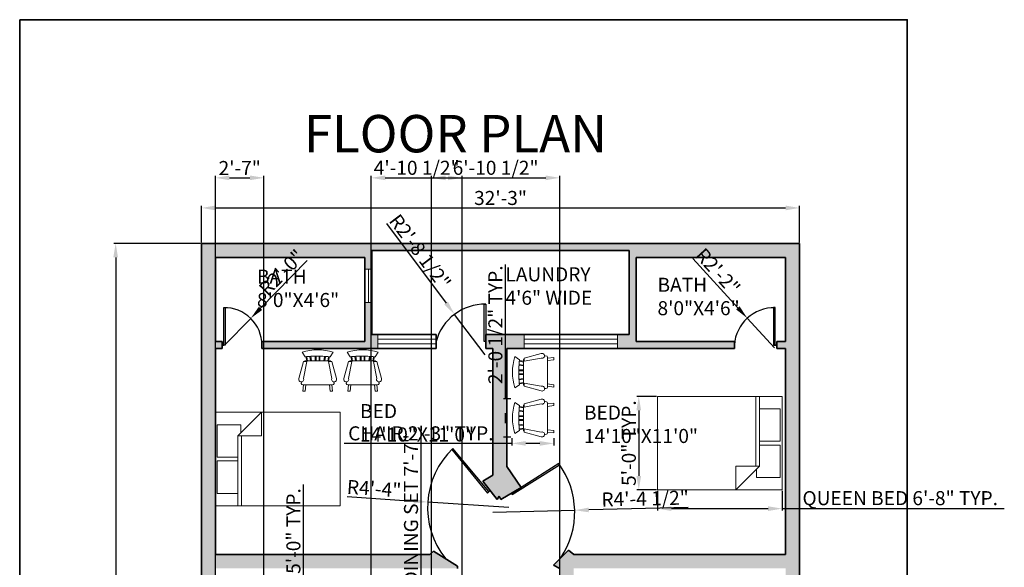
# Model space of a CAD drawing. Units: inches. Extents: x 32476 to 33108, y 58720 to 59630.
# Tile 6 of 6: x 32476 to 33108, y 59278 to 59630. Entities that reach past the tile are written whole.
import ezdxf

# ---------------------------------------------------------------- set-up
doc = ezdxf.new("R2010")
doc.units = ezdxf.units.IN
for name, color, linetype, lineweight in [('A-ANNO-DIMS', 6, 'Continuous', 18), ('A-ANNO-TTLB', 7, 'Continuous', 35), ('A-AREA-IDEN', 32, 'Continuous', 18), ('A-DOOR', 4, 'Continuous', 25), ('A-FURN', 8, 'Continuous', 18), ('A-GLAZ', 4, 'Continuous', 18), ('A-WALL', 7, 'Continuous', 35), ('A-WALL-PATT', 251, 'Continuous', 13)]:
    doc.layers.add(name, color=color, linetype=linetype, lineweight=lineweight)
doc.styles.get("Standard").update_dxf_attribs({"font": 'arial.ttf'})
doc.dimstyles.new('ISO-25', dxfattribs={"dimtxt": 9, "dimasz": 9, "dimexe": 1.25, "dimexo": 0.625, "dimtad": 1, "dimdec": 1, "dimrnd": 9, "dimlunit": 3, "dimtxsty": 'Standard', "dimcen": 2.5, "dimadec": 0, "dimazin": 0, "dimtfac": 1, "dimtdec": 1, "dimtmove": 0, "dimatfit": 3, "dimfxl": 1, "dimarcsym": 0})

# ---------------------------------------------------------------- blocks, each defined once
blk = doc.blocks.new('*D1')
at = {"layer": 'A-ANNO-DIMS', "color": 0, "lineweight": -2, "transparency": 16777216}
for p, q in [((32593.04, 59486.84), (32593.04, 59510.18)), ((32602.04, 59508.93), (32968.04, 59508.93)), ((32977.04, 59486.84), (32977.04, 59510.18))]:
    blk.add_line(p, q, dxfattribs=at)
at = {"layer": 'A-ANNO-DIMS', "color": 0, "transparency": 16777216}
for points in [[(32602.04, 59510.43), (32602.04, 59507.43), (32593.04, 59508.93)], [(32968.04, 59510.43), (32968.04, 59507.43), (32977.04, 59508.93)]]:
    blk.add_solid(points, dxfattribs=at)
at = {"layer": 'Defpoints', "color": 0, "transparency": 16777216}
for p in [(32977.04, 59508.93), (32593.04, 59486.22), (32977.04, 59486.22)]:
    blk.add_point(p, dxfattribs=at)
at = {"layer": 'A-ANNO-DIMS', "color": 0, "transparency": 16777216, "insert": (32785.04, 59514.15), "char_height": 9, "attachment_point": 5}
blk.add_mtext('32\'-3"', dxfattribs=at)
blk = doc.blocks.new('*D2')
at = {"layer": 'A-ANNO-DIMS', "color": 0, "lineweight": -2, "transparency": 16777216}
for p, q in [((32592.41, 59486.22), (32536.75, 59486.22)), ((32538, 59477.22), (32538, 58799.22)), ((32592.41, 58790.22), (32536.75, 58790.22))]:
    blk.add_line(p, q, dxfattribs=at)
at = {"layer": 'A-ANNO-DIMS', "color": 0, "transparency": 16777216}
for points in [[(32536.5, 59477.22), (32539.5, 59477.22), (32538, 59486.22)], [(32536.5, 58799.22), (32539.5, 58799.22), (32538, 58790.22)]]:
    blk.add_solid(points, dxfattribs=at)
at = {"layer": 'Defpoints', "color": 0, "transparency": 16777216}
for p in [(32593.04, 59486.22), (32538, 58790.22), (32593.04, 58790.22)]:
    blk.add_point(p, dxfattribs=at)
at = {"layer": 'A-ANNO-DIMS', "color": 0, "transparency": 16777216, "insert": (32532.78, 59138.22), "char_height": 9, "attachment_point": 5, "rotation": 90}
blk.add_mtext('57\'-9"', dxfattribs=at)
blk = doc.blocks.new('Bed - Queen')
for p, q in [((0, -80.00003), (0, 0)), ((0, 0), (59.99999, 0)), ((59.99999, 0), (59.99999, -80.00003)), ((7.99999, -1.2), (28.79998, -1.2)), ((7.99999, -14.4), (7.99999, -1.2)), ((28.79998, -1.2), (28.79998, -14.4)), ((31.19999, -1.2), (51.99999, -1.2)), ((31.19999, -14.4), (31.19999, -1.2)), ((51.99999, -1.2), (51.99999, -16.4)), ((0, -14.4), (44.8, -14.4)), ((44.8, -16.8), (0, -16.8)), ((59.99999, -29.6), (44.8, -14.4)), ((44.8, -14.4), (44.8, -29.6)), ((51.99999, -16.4), (46.79936, -16.4)), ((44.8, -29.6), (59.99999, -29.6)), ((59.99999, -80.00003), (0, -80.00003))]:
    blk.add_line(p, q)
blk = doc.blocks.new('Chair - Rocking')
for p, q in [((-8, -4.5), (-10, -1.5)), ((-7.5, -4.5), (-7, -7)), ((-6.5, -7), (-7.02225, -4.43)), ((-4.5, -7), (-4.96674, -4.19951)), ((-4, -7), (-4.40532, -4.16272)), ((-1.5, -4.05012), (-1.5, -7)), ((-1, -7), (-1, -4.05012)), ((1, -7), (1, -4.04655)), ((1.5, -4.05012), (1.5, -7)), ((4, -7), (4.40187, -4.18694)), ((4.5, -7), (4.96761, -4.19437)), ((6.5, -7), (7, -4.4057)), ((7.5, -4.5), (7, -7)), ((8, -4.5), (10, -1.5)), ((-9, -7.5), (-12, -18.49999)), ((-7, -7.5), (-9, -7.5)), ((-9, -18.49999), (-7, -7.5)), ((-8.23428, -6.99939), (-8.3093, -7.47958)), ((-8.23041, -7), (8.23915, -7)), ((7, -7.5), (9, -7.5)), ((9, -18.49999), (7, -7.5)), ((8.31071, -7.48854), (8.23449, -7.00073)), ((9, -7.5), (12, -18.49999)), ((-10.36644, -20.64523), (-10.5, -21.49999)), ((-9, -22.49999), (-9.5, -26.49999)), ((0, -22.49999), (-9.5, -22.49999)), ((-8, -26.49999), (-7.5, -22.49999)), ((0, -22.49999), (9.5, -22.49999)), ((8, -26.49999), (7.5, -22.49999)), ((9, -22.49999), (9.5, -26.49999)), ((10.5, -21.49999), (10.3575, -20.58798)), ((-9.5, -26.49999), (-8, -26.49999)), ((9.5, -26.49999), (8, -26.49999))]:
    blk.add_line(p, q)
for centre, radius, start, end in [((0, -34.08333), 34.08333, 72.93847, 107.0615), ((0, -68.25004), 64.25, 93.92211, 97.15267), ((0, -68.25004), 64.25, 82.84733, 93.92211), ((-10.5, -18.99999), 1.58114, 161.5651, 18.43495), ((10.5, -18.99999), 1.58114, 161.5651, 18.43495), ((-9.5, -21.49999), 1, 180, 270), ((9.5, -21.49999), 1, 270, 0)]:
    blk.add_arc(centre, radius, start, end)
blk = doc.blocks.new('*D15')
at = {"layer": 'A-ANNO-DIMS', "color": 0, "lineweight": -2, "transparency": 16777216}
for p, q in [((32792.22, 59361.34), (32792.22, 59356.67)), ((32819.22, 59361.34), (32819.22, 59356.67)), ((32792.22, 59357.92), (32684.61, 59357.92)), ((32810.22, 59357.92), (32801.22, 59357.92))]:
    blk.add_line(p, q, dxfattribs=at)
at = {"layer": 'A-ANNO-DIMS', "color": 0, "transparency": 16777216}
for points in [[(32801.22, 59359.42), (32801.22, 59356.42), (32792.22, 59357.92)], [(32810.22, 59359.42), (32810.22, 59356.42), (32819.22, 59357.92)]]:
    blk.add_solid(points, dxfattribs=at)
at = {"layer": 'Defpoints', "color": 0, "transparency": 16777216}
for p in [(32792.22, 59361.97), (32819.22, 59361.97), (32792.22, 59357.92)]:
    blk.add_point(p, dxfattribs=at)
at = {"layer": 'A-ANNO-DIMS', "color": 0, "transparency": 16777216, "insert": (32733.91, 59363.2), "char_height": 9, "attachment_point": 5}
blk.add_mtext('CHAIR 2\'-3" TYP.', dxfattribs=at)
blk = doc.blocks.new('*D16')
at = {"layer": 'A-ANNO-DIMS', "color": 0, "lineweight": -2, "transparency": 16777216}
for p, q in [((32788.17, 59386.4), (32788.17, 59472.64)), ((32791.6, 59386.4), (32786.92, 59386.4)), ((32788.17, 59370.97), (32788.17, 59377.4)), ((32791.6, 59361.97), (32786.92, 59361.97))]:
    blk.add_line(p, q, dxfattribs=at)
at = {"layer": 'A-ANNO-DIMS', "color": 0, "transparency": 16777216}
for points in [[(32786.67, 59377.4), (32789.67, 59377.4), (32788.17, 59386.4)], [(32786.67, 59370.97), (32789.67, 59370.97), (32788.17, 59361.97)]]:
    blk.add_solid(points, dxfattribs=at)
at = {"layer": 'Defpoints', "color": 0, "transparency": 16777216}
for p in [(32788.17, 59386.4), (32792.22, 59386.4), (32792.22, 59361.97)]:
    blk.add_point(p, dxfattribs=at)
at = {"layer": 'A-ANNO-DIMS', "color": 0, "transparency": 16777216, "insert": (32782.89, 59434.02), "char_height": 9, "attachment_point": 5, "rotation": 90}
blk.add_mtext('2\'-0 1/2" TYP.', dxfattribs=at)
blk = doc.blocks.new('*D21')
at = {"layer": 'A-ANNO-DIMS', "color": 0, "lineweight": -2, "transparency": 16777216}
for p, q in [((32885.79, 59327.47), (32885.79, 59314.84)), ((32965.79, 59327.47), (32965.79, 59314.84)), ((32894.79, 59316.09), (32956.79, 59316.09)), ((32965.79, 59316.09), (33108.43, 59316.09))]:
    blk.add_line(p, q, dxfattribs=at)
at = {"layer": 'A-ANNO-DIMS', "color": 0, "transparency": 16777216}
for points in [[(32894.79, 59317.59), (32894.79, 59314.59), (32885.79, 59316.09)], [(32956.79, 59317.59), (32956.79, 59314.59), (32965.79, 59316.09)]]:
    blk.add_solid(points, dxfattribs=at)
at = {"layer": 'Defpoints', "color": 0, "transparency": 16777216}
for p in [(32885.79, 59328.09), (32965.79, 59328.09), (32965.79, 59316.09)]:
    blk.add_point(p, dxfattribs=at)
at = {"layer": 'A-ANNO-DIMS', "color": 0, "transparency": 16777216, "insert": (33041.61, 59321.65), "char_height": 9, "attachment_point": 5}
blk.add_mtext('QUEEN BED 6\'-8" TYP.', dxfattribs=at)
blk = doc.blocks.new('*D22')
at = {"layer": 'A-ANNO-DIMS', "color": 0, "lineweight": -2, "transparency": 16777216}
for p, q in [((32885.16, 59388.09), (32872.54, 59388.09)), ((32873.79, 59379.09), (32873.79, 59337.09)), ((32885.16, 59328.09), (32872.54, 59328.09))]:
    blk.add_line(p, q, dxfattribs=at)
at = {"layer": 'A-ANNO-DIMS', "color": 0, "transparency": 16777216}
for points in [[(32872.29, 59379.09), (32875.29, 59379.09), (32873.79, 59388.09)], [(32872.29, 59337.09), (32875.29, 59337.09), (32873.79, 59328.09)]]:
    blk.add_solid(points, dxfattribs=at)
at = {"layer": 'Defpoints', "color": 0, "transparency": 16777216}
for p in [(32885.79, 59388.09), (32873.79, 59328.09), (32885.79, 59328.09)]:
    blk.add_point(p, dxfattribs=at)
at = {"layer": 'A-ANNO-DIMS', "color": 0, "transparency": 16777216, "insert": (32868.57, 59358.09), "char_height": 9, "attachment_point": 5, "rotation": 90}
blk.add_mtext('5\'-0" TYP.', dxfattribs=at)
blk = doc.blocks.new('*D25')
at = {"layer": 'A-ANNO-DIMS', "color": 0, "lineweight": -2, "transparency": 16777216}
for p, q in [((32658.53, 59229.2), (32658.53, 59331.59)), ((32666.91, 59229.2), (32657.28, 59229.2)), ((32658.53, 59178.2), (32658.53, 59220.2)), ((32666.91, 59169.2), (32657.28, 59169.2))]:
    blk.add_line(p, q, dxfattribs=at)
at = {"layer": 'A-ANNO-DIMS', "color": 0, "transparency": 16777216}
for points in [[(32657.03, 59220.2), (32660.03, 59220.2), (32658.53, 59229.2)], [(32657.03, 59178.2), (32660.03, 59178.2), (32658.53, 59169.2)]]:
    blk.add_solid(points, dxfattribs=at)
at = {"layer": 'Defpoints', "color": 0, "transparency": 16777216}
for p in [(32658.53, 59229.2), (32667.53, 59229.2), (32667.53, 59169.2)]:
    blk.add_point(p, dxfattribs=at)
at = {"layer": 'A-ANNO-DIMS', "color": 0, "transparency": 16777216, "insert": (32653.25, 59284.89), "char_height": 9, "attachment_point": 5, "rotation": 90}
blk.add_mtext('DESK 5\'-0" TYP.', dxfattribs=at)
blk = doc.blocks.new('*D31')
at = {"layer": 'A-ANNO-DIMS', "color": 0, "lineweight": -2, "transparency": 16777216}
for p, q in [((32734.02, 59256.57), (32734.02, 59365.74)), ((32747.05, 59256.57), (32732.77, 59256.57)), ((32734.02, 59174.57), (32734.02, 59247.57)), ((32747.05, 59165.57), (32732.77, 59165.57))]:
    blk.add_line(p, q, dxfattribs=at)
at = {"layer": 'A-ANNO-DIMS', "color": 0, "transparency": 16777216}
for points in [[(32732.52, 59247.57), (32735.52, 59247.57), (32734.02, 59256.57)], [(32732.52, 59174.57), (32735.52, 59174.57), (32734.02, 59165.57)]]:
    blk.add_solid(points, dxfattribs=at)
at = {"layer": 'Defpoints', "color": 0, "transparency": 16777216}
for p in [(32734.02, 59256.57), (32747.67, 59256.57), (32747.67, 59165.57)]:
    blk.add_point(p, dxfattribs=at)
at = {"layer": 'A-ANNO-DIMS', "color": 0, "transparency": 16777216, "insert": (32728.75, 59315.65), "char_height": 9, "attachment_point": 5, "rotation": 90}
blk.add_mtext('DINING SET 7\'-7"', dxfattribs=at)
blk = doc.blocks.new('*D39')
at = {"layer": 'A-ANNO-DIMS', "color": 0, "lineweight": -2, "transparency": 16777216}
for p, q in [((32702.04, 59125.34), (32702.04, 59529.47)), ((32711.04, 59528.22), (32751.42, 59528.22)), ((32760.42, 59122.05), (32760.42, 59529.47))]:
    blk.add_line(p, q, dxfattribs=at)
at = {"layer": 'A-ANNO-DIMS', "color": 0, "transparency": 16777216}
for points in [[(32711.04, 59529.72), (32711.04, 59526.72), (32702.04, 59528.22)], [(32751.42, 59529.72), (32751.42, 59526.72), (32760.42, 59528.22)]]:
    blk.add_solid(points, dxfattribs=at)
at = {"layer": 'Defpoints', "color": 0, "transparency": 16777216}
for p in [(32760.42, 59528.22), (32702.04, 59124.72), (32760.42, 59121.43)]:
    blk.add_point(p, dxfattribs=at)
at = {"layer": 'A-ANNO-DIMS', "color": 0, "transparency": 16777216, "insert": (32731.23, 59533.5), "char_height": 9, "attachment_point": 5}
blk.add_mtext('4\'-10 1/2"', dxfattribs=at)
blk = doc.blocks.new('*D41')
at = {"layer": 'A-ANNO-DIMS', "color": 0, "lineweight": -2, "transparency": 16777216}
for p, q in [((32602.04, 59125.34), (32602.04, 59529.47)), ((32611.04, 59528.22), (32624.2, 59528.22)), ((32633.2, 59125.34), (32633.2, 59529.47))]:
    blk.add_line(p, q, dxfattribs=at)
at = {"layer": 'A-ANNO-DIMS', "color": 0, "transparency": 16777216}
for points in [[(32611.04, 59529.72), (32611.04, 59526.72), (32602.04, 59528.22)], [(32624.2, 59529.72), (32624.2, 59526.72), (32633.2, 59528.22)]]:
    blk.add_solid(points, dxfattribs=at)
at = {"layer": 'Defpoints', "color": 0, "transparency": 16777216}
for p in [(32633.2, 59528.22), (32602.04, 59124.72), (32633.2, 59124.72)]:
    blk.add_point(p, dxfattribs=at)
at = {"layer": 'A-ANNO-DIMS', "color": 0, "transparency": 16777216, "insert": (32617.62, 59533.36), "char_height": 9, "attachment_point": 5}
blk.add_mtext('2\'-7"', dxfattribs=at)
blk = doc.blocks.new('*D43')
at = {"layer": 'A-ANNO-DIMS', "color": 0, "lineweight": -2, "transparency": 16777216}
for p, q in [((32740.73, 58978.34), (32740.73, 59529.47)), ((32749.73, 59528.22), (32814.04, 59528.22)), ((32823.04, 58978.34), (32823.04, 59529.47))]:
    blk.add_line(p, q, dxfattribs=at)
at = {"layer": 'A-ANNO-DIMS', "color": 0, "transparency": 16777216}
for points in [[(32749.73, 59529.72), (32749.73, 59526.72), (32740.73, 59528.22)], [(32814.04, 59529.72), (32814.04, 59526.72), (32823.04, 59528.22)]]:
    blk.add_solid(points, dxfattribs=at)
at = {"layer": 'Defpoints', "color": 0, "transparency": 16777216}
for p in [(32823.04, 59528.22), (32740.73, 58977.72), (32823.04, 58977.72)]:
    blk.add_point(p, dxfattribs=at)
at = {"layer": 'A-ANNO-DIMS', "color": 0, "transparency": 16777216, "insert": (32781.88, 59533.5), "char_height": 9, "attachment_point": 5}
blk.add_mtext('6\'-10 1/2"', dxfattribs=at)
blk = doc.blocks.new('*D50')
at = {"layer": 'A-ANNO-DIMS', "color": 0, "lineweight": -2, "transparency": 16777216}
for p, q in [((32660.92, 59475.12), (32630.98, 59444.55)), ((32607.89, 59420.96), (32624.69, 59438.12))]:
    blk.add_line(p, q, dxfattribs=at)
at = {"layer": 'A-ANNO-DIMS', "color": 0, "transparency": 16777216}
blk.add_solid([(32629.91, 59445.6), (32632.06, 59443.5), (32624.69, 59438.12)], dxfattribs=at)
at = {"layer": 'Defpoints', "color": 0, "transparency": 16777216}
for p in [(32624.69, 59438.12), (32607.89, 59420.96)]:
    blk.add_point(p, dxfattribs=at)
at = {"layer": 'A-ANNO-DIMS', "color": 0, "transparency": 16777216, "insert": (32645.37, 59466.71), "char_height": 9, "attachment_point": 5, "rotation": 45.60714}
blk.add_mtext('R2\'-0"', dxfattribs=at)
blk = doc.blocks.new('*D51')
at = {"layer": 'A-ANNO-DIMS', "color": 0, "lineweight": -2, "transparency": 16777216}
for p, q in [((32711.8, 59498.86), (32750.1, 59447.88)), ((32775.09, 59414.62), (32755.51, 59440.69))]:
    blk.add_line(p, q, dxfattribs=at)
at = {"layer": 'A-ANNO-DIMS', "color": 0, "transparency": 16777216}
blk.add_solid([(32751.3, 59448.78), (32748.9, 59446.98), (32755.51, 59440.69)], dxfattribs=at)
at = {"layer": 'Defpoints', "color": 0, "transparency": 16777216}
for p in [(32755.51, 59440.69), (32775.09, 59414.62)]:
    blk.add_point(p, dxfattribs=at)
at = {"layer": 'A-ANNO-DIMS', "color": 0, "transparency": 16777216, "insert": (32732.47, 59480.14), "char_height": 9, "attachment_point": 5, "rotation": 306.91648}
blk.add_mtext('R2\'-8 1/2"', dxfattribs=at)
blk = doc.blocks.new('*D52')
at = {"layer": 'A-ANNO-DIMS', "color": 0, "lineweight": -2, "transparency": 16777216}
for p, q in [((32908.49, 59476.41), (32937.37, 59444.85)), ((32960.86, 59419.19), (32943.45, 59438.21))]:
    blk.add_line(p, q, dxfattribs=at)
at = {"layer": 'A-ANNO-DIMS', "color": 0, "transparency": 16777216}
blk.add_solid([(32938.48, 59445.86), (32936.27, 59443.84), (32943.45, 59438.21)], dxfattribs=at)
at = {"layer": 'Defpoints', "color": 0, "transparency": 16777216}
for p in [(32943.45, 59438.21), (32960.86, 59419.19)]:
    blk.add_point(p, dxfattribs=at)
at = {"layer": 'A-ANNO-DIMS', "color": 0, "transparency": 16777216, "insert": (32923.69, 59467.42), "char_height": 9, "attachment_point": 5, "rotation": 312.46754}
blk.add_mtext('R2\'-2"', dxfattribs=at)
blk = doc.blocks.new('*D53')
at = {"layer": 'A-ANNO-DIMS', "color": 0, "lineweight": -2, "transparency": 16777216}
for p, q in [((32686.62, 59323.79), (32729.31, 59320.91)), ((32790.33, 59316.79), (32738.29, 59320.3))]:
    blk.add_line(p, q, dxfattribs=at)
at = {"layer": 'A-ANNO-DIMS', "color": 0, "transparency": 16777216}
blk.add_solid([(32729.41, 59322.41), (32729.21, 59319.41), (32738.29, 59320.3)], dxfattribs=at)
at = {"layer": 'Defpoints', "color": 0, "transparency": 16777216}
for p in [(32738.29, 59320.3), (32790.33, 59316.79)]:
    blk.add_point(p, dxfattribs=at)
at = {"layer": 'A-ANNO-DIMS', "color": 0, "transparency": 16777216, "insert": (32703.82, 59327.77), "char_height": 9, "attachment_point": 5, "rotation": 356.13615}
blk.add_mtext('R4\'-4"', dxfattribs=at)
blk = doc.blocks.new('*D54')
at = {"layer": 'A-ANNO-DIMS', "color": 0, "lineweight": -2, "transparency": 16777216}
for p, q in [((32780.14, 59313.78), (32832.66, 59315.03)), ((32905.39, 59316.77), (32841.65, 59315.25))]:
    blk.add_line(p, q, dxfattribs=at)
at = {"layer": 'A-ANNO-DIMS', "color": 0, "transparency": 16777216}
blk.add_solid([(32841.62, 59316.75), (32841.69, 59313.75), (32832.66, 59315.03)], dxfattribs=at)
at = {"layer": 'Defpoints', "color": 0, "transparency": 16777216}
for p in [(32780.14, 59313.78), (32832.66, 59315.03)]:
    blk.add_point(p, dxfattribs=at)
at = {"layer": 'A-ANNO-DIMS', "color": 0, "transparency": 16777216, "insert": (32877.9, 59321.39), "char_height": 9, "attachment_point": 5, "rotation": 1.36915}
blk.add_mtext('R4\'-4 1/2"', dxfattribs=at)

msp = doc.modelspace()

# ---------------------------------------------------------------- hatches: boundary and pattern name
at = {"layer": 'A-WALL-PATT'}
h = msp.add_hatch(color=256, dxfattribs=at)
h.dxf.hatch_style = 1
h.paths.add_polyline_path([(32602.04, 59418.72), (32606.39, 59418.72), (32606.39, 59423.22), (32602.04, 59423.22), (32602.04, 59477.22), (32698.04, 59477.22), (32698.04, 59469.73), (32702.54, 59469.73), (32702.54, 59481.72), (32867.54, 59481.72), (32867.54, 59427.72), (32860.2, 59427.72), (32860.2, 59418.72), (32867.54, 59418.72), (32935.14, 59418.72), (32935.14, 59423.22), (32872.04, 59423.22), (32872.04, 59477.22), (32968.04, 59477.22), (32968.04, 59423.22), (32962.36, 59423.22), (32962.36, 59418.72), (32968.04, 59418.72), (32968.04, 59286.72), (32867.54, 59286.72), (32832.04, 59286.72), (32828.7, 59289.44), (32818.99, 59279.82), (32823.04, 59277.72), (32823.04, 59269.52), (32832.04, 59269.52), (32832.04, 59277.72), (32867.54, 59277.72), (32968.04, 59277.72), (32968.04, 58880.22), (32925.88, 58880.22), (32925.88, 58871.22), (32968.04, 58871.22), (32968.04, 58799.22), (32823.04, 58799.22), (32823.04, 58790.22), (32977.04, 58790.22), (32977.04, 59486.22), (32867.54, 59486.22), (32702.54, 59486.22), (32593.04, 59486.22), (32593.04, 58803.66), (32602.04, 58803.66), (32602.04, 59001.72), (32624.39, 59001.72), (32624.39, 59010.72), (32602.04, 59010.72), (32602.04, 59124.72), (32648.65, 59124.72), (32648.65, 59133.72), (32602.04, 59133.72), (32602.04, 59277.72), (32757.41, 59277.72), (32757.41, 59279.22), (32742.07, 59288.84), (32739.6, 59286.72), (32702.54, 59286.72), (32602.04, 59286.72)])
h.paths.add_polyline_path([(32763.92, 59133.72), (32685.69, 59133.72), (32685.69, 59124.72), (32693.04, 59124.72), (32693.04, 59010.72), (32668.87, 59010.72), (32668.87, 59001.72), (32705.76, 59001.72), (32705.76, 59010.72), (32702.04, 59010.72), (32702.04, 59124.72), (32763.92, 59124.72)], flags=17)
h.paths.add_polyline_path([(32832.04, 59226.49), (32823.04, 59226.49), (32823.04, 59133.72), (32814.31, 59133.72), (32814.31, 59124.72), (32823.04, 59124.72), (32823.04, 59099.14), (32832.04, 59099.14), (32832.04, 59124.72), (32839.29, 59124.72), (32839.29, 59133.72), (32832.04, 59133.72)], flags=17)
h.paths.add_polyline_path([(32921.54, 59133.72), (32874.43, 59133.72), (32874.43, 59124.72), (32917.04, 59124.72), (32917.04, 59097.72), (32921.54, 59097.72), (32921.54, 59124.72)], flags=17)
h.paths.add_polyline_path([(32832.04, 59066.22), (32968.04, 59066.22), (32968.04, 59070.72), (32921.54, 59070.72), (32921.54, 59074.56), (32917.04, 59074.56), (32917.04, 59070.72), (32832.04, 59070.72), (32832.04, 59074.32), (32823.04, 59074.32), (32823.04, 59056.98), (32832.04, 59056.98)], flags=17)
h.paths.add_polyline_path([(32738.1, 59010.72), (32721.79, 59010.72), (32721.79, 59001.72), (32738.1, 59001.72)], flags=16)
h.paths.add_polyline_path([(32763.19, 59010.72), (32754.77, 59010.72), (32754.77, 59001.72), (32763.19, 59001.72)], flags=16)
h.paths.add_polyline_path([(32832.04, 59016.15), (32823.04, 59016.15), (32823.04, 59010.72), (32814.31, 59010.72), (32814.31, 59001.72), (32823.04, 59001.72), (32823.04, 58871.22), (32860.05, 58871.22), (32860.05, 58880.22), (32832.04, 58880.22)], flags=17)
h.paths.add_polyline_path([(32702.54, 59448.33), (32698.04, 59448.33), (32698.04, 59423.22), (32631.9, 59423.22), (32631.9, 59418.72), (32702.54, 59418.72), (32706.18, 59418.72), (32706.18, 59427.72), (32702.54, 59427.72)], flags=17)
h.paths.add_polyline_path([(32789.04, 59418.72), (32800.22, 59418.72), (32800.22, 59427.72), (32775.59, 59427.72), (32775.59, 59418.72), (32780.04, 59418.72), (32780.04, 59337.58), (32773.73, 59333.67), (32782.91, 59322.03), (32784.1, 59324.11), (32785.3, 59322.03), (32798.33, 59329.69), (32789.04, 59343.18)], flags=17)

# ---------------------------------------------------------------- linework, layer by layer
at = {"layer": 'A-ANNO-TTLB'}
msp.add_lwpolyline([(32476.39, 59629.64), (33046.1, 59629.64), (33046.1, 58720.03), (32476.39, 58720.03)], close=True, dxfattribs=at)
at = {"layer": 'A-DOOR'}
for p, q in [((32607.39, 59420.97), (32607.39, 59444.97)), ((32607.39, 59444.97), (32608.39, 59444.97)), ((32608.39, 59444.97), (32608.39, 59420.97)), ((32774.59, 59423.22), (32774.59, 59447.22)), ((32774.59, 59447.22), (32775.59, 59447.22)), ((32775.59, 59447.22), (32775.59, 59427.72)), ((32961.36, 59444.97), (32960.36, 59444.97)), ((32960.36, 59444.97), (32960.36, 59420.97)), ((32961.36, 59420.97), (32961.36, 59444.97)), ((32606.39, 59420.97), (32607.39, 59420.97)), ((32608.39, 59420.97), (32607.39, 59420.97)), ((32775.59, 59423.22), (32774.59, 59423.22)), ((32960.36, 59420.97), (32961.86, 59420.97)), ((32962.36, 59420.97), (32961.36, 59420.97)), ((32754.51, 59354.71), (32753.79, 59354.01)), ((32753.79, 59354.01), (32776.65, 59326.06)), ((32777.64, 59327.12), (32754.51, 59354.71)), ((32792.46, 59325.09), (32822.99, 59344.17)), ((32822.4, 59344.98), (32798.33, 59329.69)), ((32822.99, 59344.17), (32822.4, 59344.98)), ((32776.65, 59326.06), (32777.75, 59326.98)), ((32778.32, 59327.85), (32777.64, 59327.12)), ((32791.81, 59325.86), (32792.46, 59325.09))]:
    msp.add_line(p, q, dxfattribs=at)
for centre, radius, start, end in [((32607.89, 59420.96), 24.01, 0.0215, 91.19304), ((32775.09, 59414.62), 32.6, 89.12121, 164.71043), ((32960.86, 59419.19), 25.78, 88.8888, 176.04616), ((32790.33, 59316.79), 52.16, 133.36706, 218.90448), ((32780.14, 59313.78), 52.53, 326.29687, 36.44122)]:
    msp.add_arc(centre, radius, start, end, dxfattribs=at)
at = {"layer": 'A-GLAZ'}
for p, q in [((32702.54, 59469.73), (32698.04, 59469.73)), ((32700.29, 59469.73), (32700.29, 59448.33)), ((32702.54, 59448.33), (32698.04, 59448.33)), ((32706.18, 59427.72), (32706.18, 59418.72)), ((32706.18, 59424.72), (32743.64, 59424.72)), ((32800.22, 59427.72), (32800.22, 59418.72)), ((32800.22, 59424.72), (32860.2, 59424.72)), ((32860.2, 59427.72), (32860.2, 59418.72)), ((32706.18, 59421.72), (32743.64, 59421.72)), ((32800.22, 59421.72), (32860.2, 59421.72))]:
    msp.add_line(p, q, dxfattribs=at)
at = {"layer": 'A-WALL'}
for p, q in [((32593.04, 59486.22), (32593.04, 58790.22)), ((32702.54, 59486.22), (32593.04, 59486.22)), ((32702.54, 59486.22), (32867.54, 59486.22)), ((32702.54, 59481.72), (32702.54, 59427.72)), ((32702.54, 59481.72), (32867.54, 59481.72)), ((32977.04, 59486.22), (32867.54, 59486.22)), ((32867.54, 59427.72), (32867.54, 59481.72)), ((32977.04, 58790.22), (32977.04, 59486.22)), ((32602.04, 59477.22), (32602.04, 59423.22)), ((32698.04, 59477.22), (32602.04, 59477.22)), ((32698.04, 59477.22), (32698.04, 59423.22)), ((32968.04, 59477.22), (32872.04, 59477.22)), ((32872.04, 59423.22), (32872.04, 59477.22)), ((32968.04, 59423.22), (32968.04, 59477.22)), ((32702.54, 59427.72), (32743.64, 59427.72)), ((32743.64, 59427.72), (32743.64, 59418.72)), ((32775.59, 59427.72), (32775.59, 59418.72)), ((32775.59, 59427.72), (32867.54, 59427.72)), ((32606.39, 59423.22), (32602.04, 59423.22)), ((32602.04, 59418.72), (32602.04, 59286.72)), ((32606.39, 59418.72), (32602.04, 59418.72)), ((32606.39, 59423.22), (32606.39, 59418.72)), ((32698.04, 59423.22), (32631.9, 59423.22)), ((32631.9, 59423.22), (32631.9, 59418.72)), ((32702.54, 59418.72), (32631.9, 59418.72)), ((32702.54, 59418.72), (32743.64, 59418.72)), ((32775.59, 59418.72), (32780.04, 59418.72)), ((32780.04, 59418.72), (32780.04, 59337.58)), ((32789.04, 59418.72), (32789.04, 59343.18)), ((32789.04, 59418.72), (32867.54, 59418.72)), ((32935.14, 59418.72), (32867.54, 59418.72)), ((32935.14, 59423.22), (32872.04, 59423.22)), ((32935.14, 59423.22), (32935.14, 59418.72)), ((32968.04, 59423.22), (32962.36, 59423.22)), ((32962.36, 59423.22), (32962.36, 59418.72)), ((32968.04, 59418.72), (32962.36, 59418.72)), ((32968.04, 59286.72), (32968.04, 59418.72)), ((32798.33, 59329.69), (32789.04, 59343.18)), ((32780.04, 59337.58), (32773.73, 59333.67)), ((32773.73, 59333.67), (32782.91, 59322.03)), ((32782.91, 59322.03), (32784.1, 59324.11)), ((32784.1, 59324.11), (32785.3, 59322.03)), ((32785.3, 59322.03), (32798.33, 59329.69)), ((32739.6, 59286.72), (32602.04, 59286.72)), ((32702.54, 59286.72), (32739.6, 59286.72)), ((32742.07, 59288.84), (32739.6, 59286.72)), ((32757.41, 59279.22), (32742.07, 59288.84)), ((32818.99, 59279.82), (32828.7, 59289.44)), ((32828.7, 59289.44), (32832.04, 59286.72)), ((32832.04, 59286.72), (32867.54, 59286.72)), ((32968.04, 59286.72), (32867.54, 59286.72)), ((32757.41, 59277.72), (32757.41, 59279.22)), ((32823.04, 59277.72), (32818.99, 59279.82))]:
    msp.add_line(p, q, dxfattribs=at)

# ---------------------------------------------------------------- block references
at = {"layer": 'A-FURN'}
for p in [(32667.66, 59417.94), (32696.54, 59417.94)]:
    msp.add_blockref('Chair - Rocking', p, dxfattribs=at)
for name, p, rotation in [('Chair - Rocking', (32792.72, 59403.56), 90), ('Bed - Queen', (32965.79, 59388.09), 270), ('Chair - Rocking', (32792.72, 59374.19), 90), ('Bed - Queen', (32602.04, 59317.87), 89.99999999999999)]:
    msp.add_blockref(name, p, dxfattribs=dict(at, rotation=rotation))

# ---------------------------------------------------------------- texts
at = {"layer": 'A-ANNO-TTLB', "insert": (32658.79, 59568.54), "char_height": 24, "attachment_point": 1}
msp.add_mtext_dynamic_manual_height_columns('FLOOR PLAN', width=354.7501, gutter_width=12.5, heights=[0], dxfattribs=at)
at = {"layer": 'A-AREA-IDEN', "char_height": 9, "attachment_point": 1}
for s, width, insert in [('BATH\\P8\'0"X4\'6"', 57.3661, (32628.7, 59469.38)), ('LAUNDRY\\P4\'6" WIDE', 81.3126, (32788.21, 59470.84)), ('BATH\\P8\'0"X4\'6"', 57.3661, (32885.81, 59464.14)), ('BED \\P14\'10"X11\'0"', 111.7067, (32694.87, 59383.13)), ('BED\\P14\'10"X11\'0"', 91.8141, (32838.61, 59382.19))]:
    msp.add_mtext_dynamic_manual_height_columns(s, width=width, gutter_width=12.5, heights=[0], dxfattribs=dict(at, insert=insert))

# ---------------------------------------------------------------- dimensions: what is measured, and where the dimension line sits
at = {"layer": 'A-ANNO-DIMS'}
for base, p1, p2, override, picture, middle in [((32760.42, 59528.22), (32702.04, 59124.72), (32760.42, 59121.43), {"dimdec": 1, "dimlfac": 1, "dimrnd": 0, "dimzin": 1, "dimdsep": 46, "dimlunit": 4, "dimfrac": 2}, '*D39', (32731.23, 59533.5)), ((32823.04, 59528.22), (32740.73, 58977.72), (32823.04, 58977.72), {"dimdec": 1, "dimlfac": 1, "dimrnd": 0, "dimzin": 1, "dimdsep": 46, "dimlunit": 4, "dimfrac": 2}, '*D43', (32781.88, 59533.5)), ((32633.2, 59528.22), (32602.04, 59124.72), (32633.2, 59124.72), {"dimdec": 1, "dimlfac": 1, "dimrnd": 0, "dimzin": 1, "dimdsep": 46, "dimlunit": 4, "dimfrac": 2}, '*D41', (32617.62, 59533.36)), ((32977.04, 59508.93), (32593.04, 59486.22), (32977.04, 59486.22), {"dimclrd": 0, "dimclre": 0, "dimclrt": 0}, '*D1', (32785.04, 59514.15))]:
    dim = msp.add_linear_dim(base=base, p1=p1, p2=p2, dimstyle='ISO-25', override=override, dxfattribs=at)
    dim.commit()
    dim.dimension.update_dxf_attribs({"geometry": picture, "text_midpoint": middle})
for center, mpoint, picture, middle in [((32775.09, 59414.62), (32755.51, 59440.69), '*D51', (32732.47, 59480.14)), ((32607.89, 59420.96), (32624.69, 59438.12), '*D50', (32645.37, 59466.71)), ((32960.86, 59419.19), (32943.45, 59438.21), '*D52', (32923.69, 59467.42)), ((32790.33, 59316.79), (32738.29, 59320.3), '*D53', (32703.82, 59327.77)), ((32780.14, 59313.78), (32832.66, 59315.03), '*D54', (32877.9, 59321.39))]:
    dim = msp.add_radius_dim(center=center, mpoint=mpoint, dimstyle='ISO-25', override={"dimdec": 1, "dimlfac": 1, "dimrnd": 0, "dimzin": 1, "dimdsep": 46, "dimlunit": 4, "dimfrac": 2}, dxfattribs=at)
    dim.commit()
    dim.dimension.update_dxf_attribs({"geometry": picture, "text_midpoint": middle})
dim = msp.add_linear_dim(base=(32538, 58790.22), p1=(32593.04, 59486.22), p2=(32593.04, 58790.22), angle=90, dimstyle='ISO-25', override={"dimclrd": 0, "dimclre": 0, "dimclrt": 0}, dxfattribs=at)
dim.commit()
dim.dimension.update_dxf_attribs({"geometry": '*D2', "text_midpoint": (32532.78, 59138.22)})
for base, p1, p2, angle, text, picture, middle in [((32788.17, 59386.4), (32792.22, 59361.97), (32792.22, 59386.4), 90, '<> TYP.', '*D16', (32782.89, 59434.02)), ((32873.79, 59328.09), (32885.79, 59388.09), (32885.79, 59328.09), 270, '<> TYP.', '*D22', (32868.57, 59358.09)), ((32792.22, 59357.92), (32819.22, 59361.97), (32792.22, 59361.97), 180, 'CHAIR <> TYP.', '*D15', (32733.91, 59363.2)), ((32734.02, 59256.57), (32747.67, 59165.57), (32747.67, 59256.57), 90, 'DINING SET <>', '*D31', (32728.75, 59315.65)), ((32658.53, 59229.2), (32667.53, 59169.2), (32667.53, 59229.2), 90, 'DESK <> TYP.', '*D25', (32653.25, 59284.89))]:
    dim = msp.add_linear_dim(base=base, p1=p1, p2=p2, angle=angle, text=text, dimstyle='ISO-25', override={"dimdec": 1, "dimlfac": 1, "dimrnd": 0, "dimzin": 1, "dimdsep": 46, "dimlunit": 4, "dimfrac": 2}, dxfattribs=at)
    dim.commit()
    dim.dimension.update_dxf_attribs({"geometry": picture, "text_midpoint": middle})
dim = msp.add_linear_dim(base=(32965.79, 59316.09), p1=(32885.79, 59328.09), p2=(32965.79, 59328.09), text='QUEEN BED <> TYP.', dimstyle='ISO-25', override={"dimdec": 1, "dimlfac": 1, "dimrnd": 0, "dimzin": 1, "dimdsep": 46, "dimlunit": 4, "dimfrac": 2}, dxfattribs=at)
dim.commit()
dim.dimension.update_dxf_attribs({"geometry": '*D21', "text_midpoint": (33041.61, 59321.65)})

doc.saveas('drawing.dxf')
